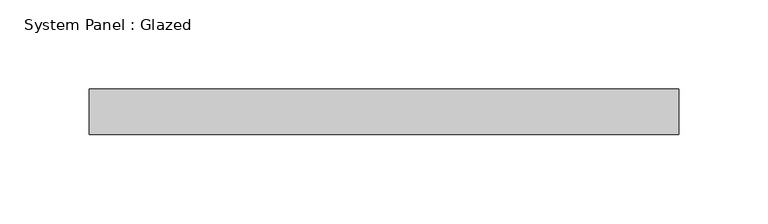
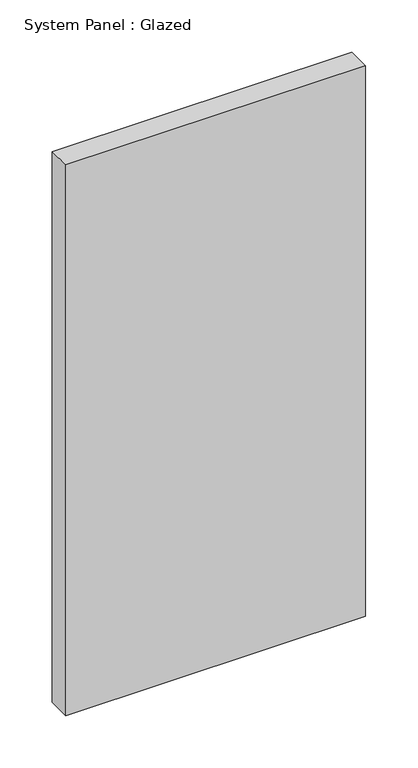
"""IFC4 building model written with IfcOpenShell, lengths in millimetres: plate geometry, System Panel : Glazed."""

from ifc_helpers import new_model, si_unit, origin, origin_with_axes, place, context, project, spatial, polyline, outline, extrude, source, transform, mapped, element, save


def system_panel_glazed_3a0990d6(model_context):
    return source(origin(), model_context, "Body", "SweptSolid", [
        extrude(outline(polyline([(165.1, 19.05), (-165.1, 19.05), (-165.1, 44.45), (165.1, 44.45), (165.1, 19.05)])), origin_with_axes(), (0.0, 0.0, 1.0), 640.9785299),
    ])


if __name__ == "__main__":
    model = new_model("IFC4")
    model_context = context("Model", 3, world=origin())
    ifc_project = project(units=[si_unit("LENGTHUNIT", "METRE", prefix="MILLI")], contexts=[model_context])
    site = spatial("IfcSite", under=ifc_project)
    building = spatial("IfcBuilding", under=site)
    placement = place(None, origin())
    system_panel_glazed_shape = system_panel_glazed_3a0990d6(model_context)
    element("IfcPlate", 1, ObjectType="System Panel : Glazed", at=placement, inside=building, context=model_context, shape_type="MappedRepresentation", body=[
        mapped(system_panel_glazed_shape, transform((0.0, 0.0, 0.0), x_axis=(1.0, 0.0, 0.0), y_axis=(0.0, 1.0, 0.0), z_axis=(0.0, 0.0, 1.0))),
    ])
    save(model, "model.ifc")

# Revit data of these elements
# Type "System Panel : Glazed"
#   Construction Type Id = "GSP4R"
#   Analytic Construction = "1/8 in Pilkington single glazing"
#   Visual Light Transmittance = 0.9
#   Solar Heat Gain Coefficient = 0.86
#   Heat Transfer Coefficient (U) = 1.18115 BTU/(h·ft²·°F)
#   Define Thermal Properties by = 1
# Element 1 (IfcPlate, "System Panel : Glazed")
#   Materials on its faces: "Glass"
# Materials
#   "Glass": class "Glass", colour RGB 0 128 192, transparency 0.75, Description = "Soda Lime Glass", Cost = 0
